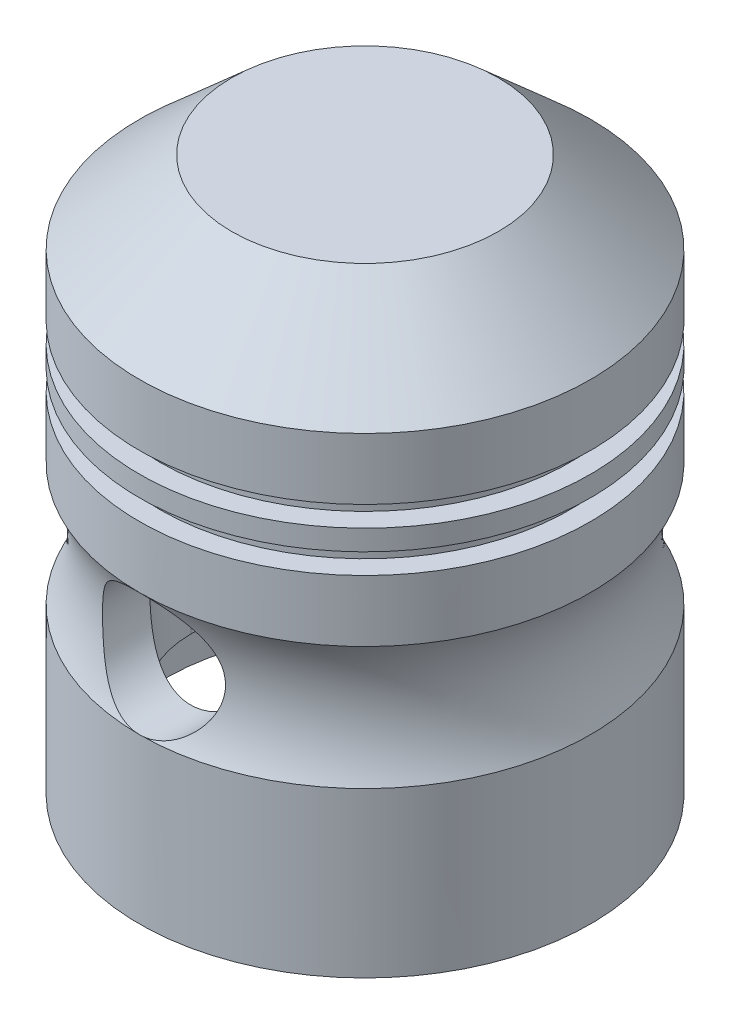
SolidWorks part; units mm, degrees
material "Plain Carbon Steel"
ref_plane "Front Plane" through (0, 0, 0) normal (0, 0, 1) x (1, 0, 0)
ref_plane "Top Plane" through (0, 0, 0) normal (0, 1, 0) x (1, 0, 0)
ref_plane "Right Plane" through (0, 0, 0) normal (1, 0, 0) x (0, 0, -1)
sketch "Piston Profile Sketch" plane through (0, 0, 0) normal (0, 0, 1) x (1, 0, 0)
  line L0 (0, -15.6437) -> (0, 20.979) construction
  line L1 (0, -12.6437) -> (11, -12.6437)
  line L2 (11, -12.6437) -> (11, -4.6437)
  line L3 (11, 1.3563) -> (11, 4.3563)
  line L4 (11, 4.3563) -> (10, 4.3563)
  line L5 (10, 4.3563) -> (10, 5.3563)
  line L6 (10, 5.3563) -> (11, 5.3563)
  line L7 (11, 5.3563) -> (11, 6.3563)
  line L8 (11, 6.3563) -> (10, 6.3563)
  line L9 (10, 6.3563) -> (10, 7.3563)
  line L10 (10, 7.3563) -> (11, 7.3563)
  line L11 (11, 7.3563) -> (11, 10.3563)
  line L12 (11, 10.3563) -> (6.5, 14.3563)
  line L13 (6.5, 14.3563) -> (0, 14.3563)
  line L14 (0, 14.3563) -> (0, -12.6437)
  arc A1 (11, 1.3563) -> (11, -4.6437) centre (16.6307, -1.6437) ccw
  dimension "D4" = 6.38
  dimension "D1" = 11
  dimension "D2" = 8
  dimension "D3" = 14
  dimension "D5" = 17
  dimension "D6" = 18
  dimension "D7" = 19
  dimension "D8" = 20
  dimension "D9" = 23
  dimension "D10" = 27
  dimension "D11" = 6.5
  dimension "D12" = 10
  dimension "D13" = 14.3563
revolve "Piston Body" add sketch "Piston Profile Sketch" angle 360 about L0
sketch "Con Rod Slot Sketch" plane through (0, -12.6437, 0) normal (0, -1, 0) x (1, 0, 0)
  line L0 (0, 11.6774) -> (0, -12.0753) construction
  line L1 (0, -3.5) -> (0, 3.5) construction
  line L2 (-5, -3.5) -> (-5, 3.5)
  line L3 (5, -3.5) -> (5, 3.5)
  arc A0 (-5, -3.5) -> (5, -3.5) centre (0, -3.5) ccw
  arc A1 (5, 3.5) -> (-5, 3.5) centre (0, 3.5) ccw
  point P5 (0, 0)
  dimension "D1" = 5
  dimension "D2" = 7
extrude "Con Rod Slot" cut sketch "Con Rod Slot Sketch" against normal blind 19
sketch "Underside Bore Sketch" plane through (0, -12.6437, 0) normal (0, -1, 0) x (1, 0, 0)
  circle A0 centre (0, 0) radius 9.75
  dimension "D1" = 19.5
extrude "Underside Bore Ø19.5" cut sketch "Underside Bore Sketch" against normal blind 6
sketch "Wrist Pin Hole Sketch" plane through (0, 0, 0) normal (0, 0, 1) x (1, 0, 0)
  line L0 (0, 18.0324) -> (0, -13.905) construction
  line L1 (-10.2507, -1.6437) -> (10.2507, -1.6437) construction
  arc A0 (-11, -4.6437) -> (-11, 1.3563) centre (-16.6307, -1.6437) ccw construction
  arc A1 (11, 1.3563) -> (11, -4.6437) centre (16.6307, -1.6437) ccw construction
  circle A2 centre (0, -1.6437) radius 3
  dimension "D1" = 6
extrude "Wrist Pin Hole Ø6" cut sketch "Wrist Pin Hole Sketch" against normal mid plane 37
